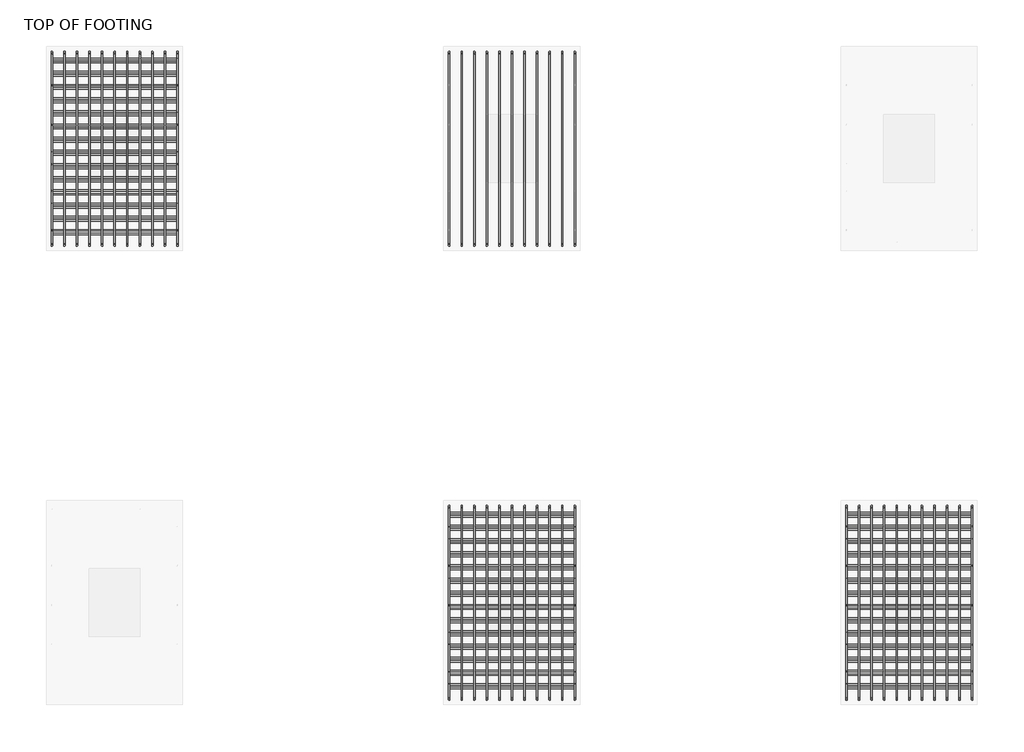
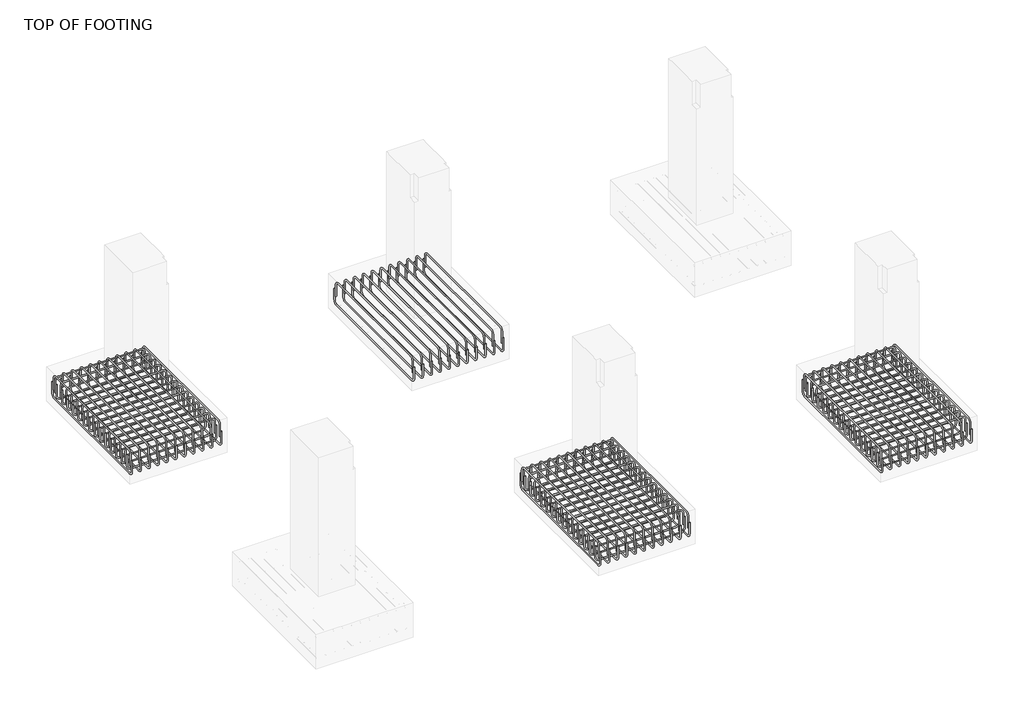
# One storey, part 5 of 11: 14 reinforcing bars.
"""IFC4 building model written with IfcOpenShell, lengths in millimetres."""

from ifc_helpers import new_model, si_unit, point, frame, origin, place, context, project, spatial, polyline, circle_curve, trimmed, segment, composite_curve, source, transform, mapped, element, save
from ifc_brep_helpers import swept_disk

model = new_model("IFC4")

# Units and contexts
model_context = context("Model", 3, world=origin())
ifc_project = project(units=[si_unit("LENGTHUNIT", "METRE", prefix="MILLI")], contexts=[model_context])

# Site, building, storey
site = spatial("IfcSite", under=ifc_project)
building = spatial("IfcBuilding", under=site)
storey = spatial("IfcBuildingStorey", under=building, Name="TOP OF FOOTING", Elevation=-1828.8)

# Reinforcing bars
placement = place(None, origin())
reinforcing_bar_shape = source(origin(), model_context, "Body", "SolidModel", [
    swept_disk(composite_curve([segment(polyline([(-8816.2384094, 14549.4712443, -2012.1658531), (-8816.2384094, 14549.4712443, -2159.4658531)]), True, "CONTINUOUS"), segment(trimmed(circle_curve(frame((-8816.2384094, 14595.8212443, -2159.4658531), z_axis=(1.0, 0.0, 0.0), x_axis=(0.0, -46.349999999998545, 0.0)), 46.35), [point((-8816.2384094, 14549.4712443, -2159.4658531))], [point((-8816.2384094, 14595.8212443, -2205.8158531))], True, "CARTESIAN"), True, "CONTINUOUS"), segment(polyline([(-8816.2384094, 14595.8212443, -2205.8158531), (-8816.2384094, 16210.4212443, -2205.8158531)]), True, "CONTINUOUS"), segment(trimmed(circle_curve(frame((-8816.2384094, 16210.4212443, -2159.4658531), z_axis=(1.0, 0.0, 0.0), x_axis=(0.0, 0.0, -46.34999999999991)), 46.35), [point((-8816.2384094, 16210.4212443, -2205.8158531))], [point((-8816.2384094, 16256.7712443, -2159.4658531))], True, "CARTESIAN"), True, "CONTINUOUS"), segment(polyline([(-8816.2384094, 16256.7712443, -2159.4658531), (-8816.2384094, 16256.7712443, -2012.1658531)]), True, "CONTINUOUS")], self_intersect=False), 6.35),
])
element("IfcReinforcingBar", 1, at=placement, inside=storey, context=model_context, shape_type="MappedRepresentation", body=[
    mapped(reinforcing_bar_shape, transform((0.0, 0.0, 0.0), x_axis=(1.0, 0.0, 0.0), y_axis=(0.0, 1.0, 0.0), z_axis=(0.0, 0.0, 1.0))),
    mapped(reinforcing_bar_shape, transform((-110.73, 0.0, 0.0), x_axis=(1.0, 0.0, 0.0), y_axis=(0.0, 1.0, 0.0), z_axis=(0.0, 0.0, 1.0))),
    mapped(reinforcing_bar_shape, transform((-221.46, 0.0, 0.0), x_axis=(1.0, 0.0, 0.0), y_axis=(0.0, 1.0, 0.0), z_axis=(0.0, 0.0, 1.0))),
    mapped(reinforcing_bar_shape, transform((-332.19, 0.0, 0.0), x_axis=(1.0, 0.0, 0.0), y_axis=(0.0, 1.0, 0.0), z_axis=(0.0, 0.0, 1.0))),
    mapped(reinforcing_bar_shape, transform((-442.92, 0.0, 0.0), x_axis=(1.0, 0.0, 0.0), y_axis=(0.0, 1.0, 0.0), z_axis=(0.0, 0.0, 1.0))),
    mapped(reinforcing_bar_shape, transform((-553.65, 0.0, 0.0), x_axis=(1.0, 0.0, 0.0), y_axis=(0.0, 1.0, 0.0), z_axis=(0.0, 0.0, 1.0))),
    mapped(reinforcing_bar_shape, transform((-664.38, 0.0, 0.0), x_axis=(1.0, 0.0, 0.0), y_axis=(0.0, 1.0, 0.0), z_axis=(0.0, 0.0, 1.0))),
    mapped(reinforcing_bar_shape, transform((-775.11, 0.0, 0.0), x_axis=(1.0, 0.0, 0.0), y_axis=(0.0, 1.0, 0.0), z_axis=(0.0, 0.0, 1.0))),
    mapped(reinforcing_bar_shape, transform((-885.84, 0.0, 0.0), x_axis=(1.0, 0.0, 0.0), y_axis=(0.0, 1.0, 0.0), z_axis=(0.0, 0.0, 1.0))),
    mapped(reinforcing_bar_shape, transform((-996.57, 0.0, 0.0), x_axis=(1.0, 0.0, 0.0), y_axis=(0.0, 1.0, 0.0), z_axis=(0.0, 0.0, 1.0))),
    mapped(reinforcing_bar_shape, transform((-1107.3, 0.0, 0.0), x_axis=(1.0, 0.0, 0.0), y_axis=(0.0, 1.0, 0.0), z_axis=(0.0, 0.0, 1.0))),
])
reinforcing_bar_2_shape = source(origin(), model_context, "Body", "SolidModel", [
    swept_disk(composite_curve([segment(polyline([(-9923.5384094, 14577.6603603, -2096.8914539), (-9923.5384094, 14577.6603603, -1949.5914539)]), True, "CONTINUOUS"), segment(trimmed(circle_curve(frame((-9923.5384094, 14624.0103603, -1949.5914539), z_axis=(-1.0, 0.0, 0.0), x_axis=(0.0, -46.350000000000364, 0.0)), 46.35), [point((-9923.5384094, 14577.6603603, -1949.5914539))], [point((-9923.5384094, 14624.0103603, -1903.2414539))], True, "CARTESIAN"), True, "CONTINUOUS"), segment(polyline([(-9923.5384094, 14624.0103603, -1903.2414539), (-9923.5384094, 16181.3238837, -1903.2414539)]), True, "CONTINUOUS"), segment(trimmed(circle_curve(frame((-9923.5384094, 16181.3238837, -1949.5914539), z_axis=(-1.0, 0.0, 0.0), x_axis=(0.0, 0.0, 46.350000000000136)), 46.35), [point((-9923.5384094, 16181.3238837, -1903.2414539))], [point((-9923.5384094, 16227.6738837, -1949.5914539))], True, "CARTESIAN"), True, "CONTINUOUS"), segment(polyline([(-9923.5384094, 16227.6738837, -1949.5914539), (-9923.5384094, 16227.6738837, -2096.8914539)]), True, "CONTINUOUS")], self_intersect=False), 6.35),
])
element("IfcReinforcingBar", 2, at=placement, inside=storey, context=model_context, shape_type="MappedRepresentation", body=[
    mapped(reinforcing_bar_2_shape, transform((0.0, 0.0, 0.0), x_axis=(1.0, 0.0, 0.0), y_axis=(0.0, 1.0, 0.0), z_axis=(0.0, 0.0, 1.0))),
    mapped(reinforcing_bar_2_shape, transform((110.73, 0.0, 0.0), x_axis=(1.0, 0.0, 0.0), y_axis=(0.0, 1.0, 0.0), z_axis=(0.0, 0.0, 1.0))),
    mapped(reinforcing_bar_2_shape, transform((221.46, 0.0, 0.0), x_axis=(1.0, 0.0, 0.0), y_axis=(0.0, 1.0, 0.0), z_axis=(0.0, 0.0, 1.0))),
    mapped(reinforcing_bar_2_shape, transform((332.19, 0.0, 0.0), x_axis=(1.0, 0.0, 0.0), y_axis=(0.0, 1.0, 0.0), z_axis=(0.0, 0.0, 1.0))),
    mapped(reinforcing_bar_2_shape, transform((442.92, 0.0, 0.0), x_axis=(1.0, 0.0, 0.0), y_axis=(0.0, 1.0, 0.0), z_axis=(0.0, 0.0, 1.0))),
    mapped(reinforcing_bar_2_shape, transform((553.65, 0.0, 0.0), x_axis=(1.0, 0.0, 0.0), y_axis=(0.0, 1.0, 0.0), z_axis=(0.0, 0.0, 1.0))),
    mapped(reinforcing_bar_2_shape, transform((664.38, 0.0, 0.0), x_axis=(1.0, 0.0, 0.0), y_axis=(0.0, 1.0, 0.0), z_axis=(0.0, 0.0, 1.0))),
    mapped(reinforcing_bar_2_shape, transform((775.11, 0.0, 0.0), x_axis=(1.0, 0.0, 0.0), y_axis=(0.0, 1.0, 0.0), z_axis=(0.0, 0.0, 1.0))),
    mapped(reinforcing_bar_2_shape, transform((885.84, 0.0, 0.0), x_axis=(1.0, 0.0, 0.0), y_axis=(0.0, 1.0, 0.0), z_axis=(0.0, 0.0, 1.0))),
    mapped(reinforcing_bar_2_shape, transform((996.57, 0.0, 0.0), x_axis=(1.0, 0.0, 0.0), y_axis=(0.0, 1.0, 0.0), z_axis=(0.0, 0.0, 1.0))),
    mapped(reinforcing_bar_2_shape, transform((1107.3, 0.0, 0.0), x_axis=(1.0, 0.0, 0.0), y_axis=(0.0, 1.0, 0.0), z_axis=(0.0, 0.0, 1.0))),
])
reinforcing_bar_3_shape = source(origin(), model_context, "Body", "SolidModel", [
    swept_disk(composite_curve([segment(polyline([(-9923.5384094, 14653.1930221, -1996.7664426), (-9923.5384094, 14653.1930221, -2144.0664426)]), True, "CONTINUOUS"), segment(trimmed(circle_curve(frame((-9877.1884094, 14653.1930221, -2144.0664426), z_axis=(0.0, -1.0, 0.0), x_axis=(-46.350000000000364, 0.0, 0.0)), 46.35), [point((-9923.5384094, 14653.1930221, -2144.0664426))], [point((-9877.1884094, 14653.1930221, -2190.4164426))], True, "CARTESIAN"), True, "CONTINUOUS"), segment(polyline([(-9877.1884094, 14653.1930221, -2190.4164426), (-8862.5884094, 14653.1930221, -2190.4164426)]), True, "CONTINUOUS"), segment(trimmed(circle_curve(frame((-8862.5884094, 14653.1930221, -2144.0664426), z_axis=(0.0, -1.0, 0.0), x_axis=(0.0, 0.0, -46.350000000000364)), 46.35), [point((-8862.5884094, 14653.1930221, -2190.4164426))], [point((-8816.2384094, 14653.1930221, -2144.0664426))], True, "CARTESIAN"), True, "CONTINUOUS"), segment(polyline([(-8816.2384094, 14653.1930221, -2144.0664426), (-8816.2384094, 14653.1930221, -1996.7664426)]), True, "CONTINUOUS")], self_intersect=False), 6.35),
])
element("IfcReinforcingBar", 3, at=placement, inside=storey, context=model_context, shape_type="MappedRepresentation", body=[
    mapped(reinforcing_bar_3_shape, transform((0.0, 0.0, 0.0), x_axis=(1.0, 0.0, 0.0), y_axis=(0.0, 1.0, 0.0), z_axis=(0.0, 0.0, 1.0))),
    mapped(reinforcing_bar_3_shape, transform((0.0, 116.2744005, 0.0), x_axis=(1.0, 0.0, 0.0), y_axis=(0.0, 1.0, 0.0), z_axis=(0.0, 0.0, 1.0))),
    mapped(reinforcing_bar_3_shape, transform((0.0, 232.5488009, 0.0), x_axis=(1.0, 0.0, 0.0), y_axis=(0.0, 1.0, 0.0), z_axis=(0.0, 0.0, 1.0))),
    mapped(reinforcing_bar_3_shape, transform((0.0, 348.8232014, 0.0), x_axis=(1.0, 0.0, 0.0), y_axis=(0.0, 1.0, 0.0), z_axis=(0.0, 0.0, 1.0))),
    mapped(reinforcing_bar_3_shape, transform((0.0, 465.0976018, 0.0), x_axis=(1.0, 0.0, 0.0), y_axis=(0.0, 1.0, 0.0), z_axis=(0.0, 0.0, 1.0))),
    mapped(reinforcing_bar_3_shape, transform((0.0, 581.3720023, 0.0), x_axis=(1.0, 0.0, 0.0), y_axis=(0.0, 1.0, 0.0), z_axis=(0.0, 0.0, 1.0))),
    mapped(reinforcing_bar_3_shape, transform((0.0, 697.6464027, 0.0), x_axis=(1.0, 0.0, 0.0), y_axis=(0.0, 1.0, 0.0), z_axis=(0.0, 0.0, 1.0))),
    mapped(reinforcing_bar_3_shape, transform((0.0, 813.9208032, 0.0), x_axis=(1.0, 0.0, 0.0), y_axis=(0.0, 1.0, 0.0), z_axis=(0.0, 0.0, 1.0))),
    mapped(reinforcing_bar_3_shape, transform((0.0, 930.1952036, 0.0), x_axis=(1.0, 0.0, 0.0), y_axis=(0.0, 1.0, 0.0), z_axis=(0.0, 0.0, 1.0))),
    mapped(reinforcing_bar_3_shape, transform((0.0, 1046.4696041, 0.0), x_axis=(1.0, 0.0, 0.0), y_axis=(0.0, 1.0, 0.0), z_axis=(0.0, 0.0, 1.0))),
    mapped(reinforcing_bar_3_shape, transform((0.0, 1162.7440045, 0.0), x_axis=(1.0, 0.0, 0.0), y_axis=(0.0, 1.0, 0.0), z_axis=(0.0, 0.0, 1.0))),
    mapped(reinforcing_bar_3_shape, transform((0.0, 1279.018405, 0.0), x_axis=(1.0, 0.0, 0.0), y_axis=(0.0, 1.0, 0.0), z_axis=(0.0, 0.0, 1.0))),
    mapped(reinforcing_bar_3_shape, transform((0.0, 1395.2928054, 0.0), x_axis=(1.0, 0.0, 0.0), y_axis=(0.0, 1.0, 0.0), z_axis=(0.0, 0.0, 1.0))),
    mapped(reinforcing_bar_3_shape, transform((0.0, 1511.5672059, 0.0), x_axis=(1.0, 0.0, 0.0), y_axis=(0.0, 1.0, 0.0), z_axis=(0.0, 0.0, 1.0))),
])
reinforcing_bar_4_shape = source(origin(), model_context, "Body", "SolidModel", [
    swept_disk(composite_curve([segment(polyline([(-9923.5384094, 16194.4257435, -2114.1958609), (-9923.5384094, 16194.4257435, -1966.8958609)]), True, "CONTINUOUS"), segment(trimmed(circle_curve(frame((-9877.1884094, 16194.4257435, -1966.8958609), z_axis=(0.0, 1.0, 0.0), x_axis=(-46.350000000000364, 0.0, 0.0)), 46.35), [point((-9923.5384094, 16194.4257435, -1966.8958609))], [point((-9877.1884094, 16194.4257435, -1920.5458609))], True, "CARTESIAN"), True, "CONTINUOUS"), segment(polyline([(-9877.1884094, 16194.4257435, -1920.5458609), (-8862.5884094, 16194.4257435, -1920.5458609)]), True, "CONTINUOUS"), segment(trimmed(circle_curve(frame((-8862.5884094, 16194.4257435, -1966.8958609), z_axis=(0.0, 1.0, 0.0), x_axis=(0.0, 0.0, 46.34999999999991)), 46.35), [point((-8862.5884094, 16194.4257435, -1920.5458609))], [point((-8816.2384094, 16194.4257435, -1966.8958609))], True, "CARTESIAN"), True, "CONTINUOUS"), segment(polyline([(-8816.2384094, 16194.4257435, -1966.8958609), (-8816.2384094, 16194.4257435, -2114.1958609)]), True, "CONTINUOUS")], self_intersect=False), 6.35),
])
element("IfcReinforcingBar", 4, at=placement, inside=storey, context=model_context, shape_type="MappedRepresentation", body=[
    mapped(reinforcing_bar_4_shape, transform((0.0, 0.0, 0.0), x_axis=(1.0, 0.0, 0.0), y_axis=(0.0, 1.0, 0.0), z_axis=(0.0, 0.0, 1.0))),
    mapped(reinforcing_bar_4_shape, transform((0.0, -116.1057918, 0.0), x_axis=(1.0, 0.0, 0.0), y_axis=(0.0, 1.0, 0.0), z_axis=(0.0, 0.0, 1.0))),
    mapped(reinforcing_bar_4_shape, transform((0.0, -232.2115836, 0.0), x_axis=(1.0, 0.0, 0.0), y_axis=(0.0, 1.0, 0.0), z_axis=(0.0, 0.0, 1.0))),
    mapped(reinforcing_bar_4_shape, transform((0.0, -348.3173754, 0.0), x_axis=(1.0, 0.0, 0.0), y_axis=(0.0, 1.0, 0.0), z_axis=(0.0, 0.0, 1.0))),
    mapped(reinforcing_bar_4_shape, transform((0.0, -464.4231672, 0.0), x_axis=(1.0, 0.0, 0.0), y_axis=(0.0, 1.0, 0.0), z_axis=(0.0, 0.0, 1.0))),
    mapped(reinforcing_bar_4_shape, transform((0.0, -580.528959, 0.0), x_axis=(1.0, 0.0, 0.0), y_axis=(0.0, 1.0, 0.0), z_axis=(0.0, 0.0, 1.0))),
    mapped(reinforcing_bar_4_shape, transform((0.0, -696.6347508, 0.0), x_axis=(1.0, 0.0, 0.0), y_axis=(0.0, 1.0, 0.0), z_axis=(0.0, 0.0, 1.0))),
    mapped(reinforcing_bar_4_shape, transform((0.0, -812.7405426, 0.0), x_axis=(1.0, 0.0, 0.0), y_axis=(0.0, 1.0, 0.0), z_axis=(0.0, 0.0, 1.0))),
    mapped(reinforcing_bar_4_shape, transform((0.0, -928.8463344, 0.0), x_axis=(1.0, 0.0, 0.0), y_axis=(0.0, 1.0, 0.0), z_axis=(0.0, 0.0, 1.0))),
    mapped(reinforcing_bar_4_shape, transform((0.0, -1044.9521262, 0.0), x_axis=(1.0, 0.0, 0.0), y_axis=(0.0, 1.0, 0.0), z_axis=(0.0, 0.0, 1.0))),
    mapped(reinforcing_bar_4_shape, transform((0.0, -1161.057918, 0.0), x_axis=(1.0, 0.0, 0.0), y_axis=(0.0, 1.0, 0.0), z_axis=(0.0, 0.0, 1.0))),
    mapped(reinforcing_bar_4_shape, transform((0.0, -1277.1637098, 0.0), x_axis=(1.0, 0.0, 0.0), y_axis=(0.0, 1.0, 0.0), z_axis=(0.0, 0.0, 1.0))),
    mapped(reinforcing_bar_4_shape, transform((0.0, -1393.2695016, 0.0), x_axis=(1.0, 0.0, 0.0), y_axis=(0.0, 1.0, 0.0), z_axis=(0.0, 0.0, 1.0))),
    mapped(reinforcing_bar_4_shape, transform((0.0, -1509.3752934, 0.0), x_axis=(1.0, 0.0, 0.0), y_axis=(0.0, 1.0, 0.0), z_axis=(0.0, 0.0, 1.0))),
])
reinforcing_bar_5_shape = source(origin(), model_context, "Body", "SolidModel", [
    swept_disk(composite_curve([segment(polyline([(-5316.2384094, 14549.4712443, -2012.1658531), (-5316.2384094, 14549.4712443, -2159.4658531)]), True, "CONTINUOUS"), segment(trimmed(circle_curve(frame((-5316.2384094, 14595.8212443, -2159.4658531), z_axis=(1.0, 0.0, 0.0), x_axis=(0.0, -46.349999999998545, 0.0)), 46.35), [point((-5316.2384094, 14549.4712443, -2159.4658531))], [point((-5316.2384094, 14595.8212443, -2205.8158531))], True, "CARTESIAN"), True, "CONTINUOUS"), segment(polyline([(-5316.2384094, 14595.8212443, -2205.8158531), (-5316.2384094, 16210.4212443, -2205.8158531)]), True, "CONTINUOUS"), segment(trimmed(circle_curve(frame((-5316.2384094, 16210.4212443, -2159.4658531), z_axis=(1.0, 0.0, 0.0), x_axis=(0.0, 0.0, -46.34999999999991)), 46.35), [point((-5316.2384094, 16210.4212443, -2205.8158531))], [point((-5316.2384094, 16256.7712443, -2159.4658531))], True, "CARTESIAN"), True, "CONTINUOUS"), segment(polyline([(-5316.2384094, 16256.7712443, -2159.4658531), (-5316.2384094, 16256.7712443, -2012.1658531)]), True, "CONTINUOUS")], self_intersect=False), 6.35),
])
element("IfcReinforcingBar", 5, at=placement, inside=storey, context=model_context, shape_type="MappedRepresentation", body=[
    mapped(reinforcing_bar_5_shape, transform((0.0, 0.0, 0.0), x_axis=(1.0, 0.0, 0.0), y_axis=(0.0, 1.0, 0.0), z_axis=(0.0, 0.0, 1.0))),
    mapped(reinforcing_bar_5_shape, transform((-110.73, 0.0, 0.0), x_axis=(1.0, 0.0, 0.0), y_axis=(0.0, 1.0, 0.0), z_axis=(0.0, 0.0, 1.0))),
    mapped(reinforcing_bar_5_shape, transform((-221.46, 0.0, 0.0), x_axis=(1.0, 0.0, 0.0), y_axis=(0.0, 1.0, 0.0), z_axis=(0.0, 0.0, 1.0))),
    mapped(reinforcing_bar_5_shape, transform((-332.19, 0.0, 0.0), x_axis=(1.0, 0.0, 0.0), y_axis=(0.0, 1.0, 0.0), z_axis=(0.0, 0.0, 1.0))),
    mapped(reinforcing_bar_5_shape, transform((-442.92, 0.0, 0.0), x_axis=(1.0, 0.0, 0.0), y_axis=(0.0, 1.0, 0.0), z_axis=(0.0, 0.0, 1.0))),
    mapped(reinforcing_bar_5_shape, transform((-553.65, 0.0, 0.0), x_axis=(1.0, 0.0, 0.0), y_axis=(0.0, 1.0, 0.0), z_axis=(0.0, 0.0, 1.0))),
    mapped(reinforcing_bar_5_shape, transform((-664.38, 0.0, 0.0), x_axis=(1.0, 0.0, 0.0), y_axis=(0.0, 1.0, 0.0), z_axis=(0.0, 0.0, 1.0))),
    mapped(reinforcing_bar_5_shape, transform((-775.11, 0.0, 0.0), x_axis=(1.0, 0.0, 0.0), y_axis=(0.0, 1.0, 0.0), z_axis=(0.0, 0.0, 1.0))),
    mapped(reinforcing_bar_5_shape, transform((-885.84, 0.0, 0.0), x_axis=(1.0, 0.0, 0.0), y_axis=(0.0, 1.0, 0.0), z_axis=(0.0, 0.0, 1.0))),
    mapped(reinforcing_bar_5_shape, transform((-996.57, 0.0, 0.0), x_axis=(1.0, 0.0, 0.0), y_axis=(0.0, 1.0, 0.0), z_axis=(0.0, 0.0, 1.0))),
    mapped(reinforcing_bar_5_shape, transform((-1107.3, 0.0, 0.0), x_axis=(1.0, 0.0, 0.0), y_axis=(0.0, 1.0, 0.0), z_axis=(0.0, 0.0, 1.0))),
])
reinforcing_bar_6_shape = source(origin(), model_context, "Body", "SolidModel", [
    swept_disk(composite_curve([segment(polyline([(-6423.5384094, 14577.6603603, -2096.8914539), (-6423.5384094, 14577.6603603, -1949.5914539)]), True, "CONTINUOUS"), segment(trimmed(circle_curve(frame((-6423.5384094, 14624.0103603, -1949.5914539), z_axis=(-1.0, 0.0, 0.0), x_axis=(0.0, -46.350000000000364, 0.0)), 46.35), [point((-6423.5384094, 14577.6603603, -1949.5914539))], [point((-6423.5384094, 14624.0103603, -1903.2414539))], True, "CARTESIAN"), True, "CONTINUOUS"), segment(polyline([(-6423.5384094, 14624.0103603, -1903.2414539), (-6423.5384094, 16181.3238837, -1903.2414539)]), True, "CONTINUOUS"), segment(trimmed(circle_curve(frame((-6423.5384094, 16181.3238837, -1949.5914539), z_axis=(-1.0, 0.0, 0.0), x_axis=(0.0, 0.0, 46.350000000000136)), 46.35), [point((-6423.5384094, 16181.3238837, -1903.2414539))], [point((-6423.5384094, 16227.6738837, -1949.5914539))], True, "CARTESIAN"), True, "CONTINUOUS"), segment(polyline([(-6423.5384094, 16227.6738837, -1949.5914539), (-6423.5384094, 16227.6738837, -2096.8914539)]), True, "CONTINUOUS")], self_intersect=False), 6.35),
])
element("IfcReinforcingBar", 6, at=placement, inside=storey, context=model_context, shape_type="MappedRepresentation", body=[
    mapped(reinforcing_bar_6_shape, transform((0.0, 0.0, 0.0), x_axis=(1.0, 0.0, 0.0), y_axis=(0.0, 1.0, 0.0), z_axis=(0.0, 0.0, 1.0))),
    mapped(reinforcing_bar_6_shape, transform((110.73, 0.0, 0.0), x_axis=(1.0, 0.0, 0.0), y_axis=(0.0, 1.0, 0.0), z_axis=(0.0, 0.0, 1.0))),
    mapped(reinforcing_bar_6_shape, transform((221.46, 0.0, 0.0), x_axis=(1.0, 0.0, 0.0), y_axis=(0.0, 1.0, 0.0), z_axis=(0.0, 0.0, 1.0))),
    mapped(reinforcing_bar_6_shape, transform((332.19, 0.0, 0.0), x_axis=(1.0, 0.0, 0.0), y_axis=(0.0, 1.0, 0.0), z_axis=(0.0, 0.0, 1.0))),
    mapped(reinforcing_bar_6_shape, transform((442.92, 0.0, 0.0), x_axis=(1.0, 0.0, 0.0), y_axis=(0.0, 1.0, 0.0), z_axis=(0.0, 0.0, 1.0))),
    mapped(reinforcing_bar_6_shape, transform((553.65, 0.0, 0.0), x_axis=(1.0, 0.0, 0.0), y_axis=(0.0, 1.0, 0.0), z_axis=(0.0, 0.0, 1.0))),
    mapped(reinforcing_bar_6_shape, transform((664.38, 0.0, 0.0), x_axis=(1.0, 0.0, 0.0), y_axis=(0.0, 1.0, 0.0), z_axis=(0.0, 0.0, 1.0))),
    mapped(reinforcing_bar_6_shape, transform((775.11, 0.0, 0.0), x_axis=(1.0, 0.0, 0.0), y_axis=(0.0, 1.0, 0.0), z_axis=(0.0, 0.0, 1.0))),
    mapped(reinforcing_bar_6_shape, transform((885.84, 0.0, 0.0), x_axis=(1.0, 0.0, 0.0), y_axis=(0.0, 1.0, 0.0), z_axis=(0.0, 0.0, 1.0))),
    mapped(reinforcing_bar_6_shape, transform((996.57, 0.0, 0.0), x_axis=(1.0, 0.0, 0.0), y_axis=(0.0, 1.0, 0.0), z_axis=(0.0, 0.0, 1.0))),
    mapped(reinforcing_bar_6_shape, transform((1107.3, 0.0, 0.0), x_axis=(1.0, 0.0, 0.0), y_axis=(0.0, 1.0, 0.0), z_axis=(0.0, 0.0, 1.0))),
])
reinforcing_bar_7_shape = source(origin(), model_context, "Body", "SolidModel", [
    swept_disk(composite_curve([segment(polyline([(-1816.2384094, 10549.4712443, -2012.1658531), (-1816.2384094, 10549.4712443, -2159.4658531)]), True, "CONTINUOUS"), segment(trimmed(circle_curve(frame((-1816.2384094, 10595.8212443, -2159.4658531), z_axis=(1.0, 0.0, 0.0), x_axis=(0.0, -46.349999999998545, 0.0)), 46.35), [point((-1816.2384094, 10549.4712443, -2159.4658531))], [point((-1816.2384094, 10595.8212443, -2205.8158531))], True, "CARTESIAN"), True, "CONTINUOUS"), segment(polyline([(-1816.2384094, 10595.8212443, -2205.8158531), (-1816.2384094, 12210.4212443, -2205.8158531)]), True, "CONTINUOUS"), segment(trimmed(circle_curve(frame((-1816.2384094, 12210.4212443, -2159.4658531), z_axis=(1.0, 0.0, 0.0), x_axis=(0.0, 0.0, -46.34999999999991)), 46.35), [point((-1816.2384094, 12210.4212443, -2205.8158531))], [point((-1816.2384094, 12256.7712443, -2159.4658531))], True, "CARTESIAN"), True, "CONTINUOUS"), segment(polyline([(-1816.2384094, 12256.7712443, -2159.4658531), (-1816.2384094, 12256.7712443, -2012.1658531)]), True, "CONTINUOUS")], self_intersect=False), 6.35),
])
element("IfcReinforcingBar", 7, at=placement, inside=storey, context=model_context, shape_type="MappedRepresentation", body=[
    mapped(reinforcing_bar_7_shape, transform((0.0, 0.0, 0.0), x_axis=(1.0, 0.0, 0.0), y_axis=(0.0, 1.0, 0.0), z_axis=(0.0, 0.0, 1.0))),
    mapped(reinforcing_bar_7_shape, transform((-110.73, 0.0, 0.0), x_axis=(1.0, 0.0, 0.0), y_axis=(0.0, 1.0, 0.0), z_axis=(0.0, 0.0, 1.0))),
    mapped(reinforcing_bar_7_shape, transform((-221.46, 0.0, 0.0), x_axis=(1.0, 0.0, 0.0), y_axis=(0.0, 1.0, 0.0), z_axis=(0.0, 0.0, 1.0))),
    mapped(reinforcing_bar_7_shape, transform((-332.19, 0.0, 0.0), x_axis=(1.0, 0.0, 0.0), y_axis=(0.0, 1.0, 0.0), z_axis=(0.0, 0.0, 1.0))),
    mapped(reinforcing_bar_7_shape, transform((-442.92, 0.0, 0.0), x_axis=(1.0, 0.0, 0.0), y_axis=(0.0, 1.0, 0.0), z_axis=(0.0, 0.0, 1.0))),
    mapped(reinforcing_bar_7_shape, transform((-553.65, 0.0, 0.0), x_axis=(1.0, 0.0, 0.0), y_axis=(0.0, 1.0, 0.0), z_axis=(0.0, 0.0, 1.0))),
    mapped(reinforcing_bar_7_shape, transform((-664.38, 0.0, 0.0), x_axis=(1.0, 0.0, 0.0), y_axis=(0.0, 1.0, 0.0), z_axis=(0.0, 0.0, 1.0))),
    mapped(reinforcing_bar_7_shape, transform((-775.11, 0.0, 0.0), x_axis=(1.0, 0.0, 0.0), y_axis=(0.0, 1.0, 0.0), z_axis=(0.0, 0.0, 1.0))),
    mapped(reinforcing_bar_7_shape, transform((-885.84, 0.0, 0.0), x_axis=(1.0, 0.0, 0.0), y_axis=(0.0, 1.0, 0.0), z_axis=(0.0, 0.0, 1.0))),
    mapped(reinforcing_bar_7_shape, transform((-996.57, 0.0, 0.0), x_axis=(1.0, 0.0, 0.0), y_axis=(0.0, 1.0, 0.0), z_axis=(0.0, 0.0, 1.0))),
    mapped(reinforcing_bar_7_shape, transform((-1107.3, 0.0, 0.0), x_axis=(1.0, 0.0, 0.0), y_axis=(0.0, 1.0, 0.0), z_axis=(0.0, 0.0, 1.0))),
])
reinforcing_bar_8_shape = source(origin(), model_context, "Body", "SolidModel", [
    swept_disk(composite_curve([segment(polyline([(-2923.5384094, 10577.6603603, -2096.8914539), (-2923.5384094, 10577.6603603, -1949.5914539)]), True, "CONTINUOUS"), segment(trimmed(circle_curve(frame((-2923.5384094, 10624.0103603, -1949.5914539), z_axis=(-1.0, 0.0, 0.0), x_axis=(0.0, -46.350000000000364, 0.0)), 46.35), [point((-2923.5384094, 10577.6603603, -1949.5914539))], [point((-2923.5384094, 10624.0103603, -1903.2414539))], True, "CARTESIAN"), True, "CONTINUOUS"), segment(polyline([(-2923.5384094, 10624.0103603, -1903.2414539), (-2923.5384094, 12181.3238837, -1903.2414539)]), True, "CONTINUOUS"), segment(trimmed(circle_curve(frame((-2923.5384094, 12181.3238837, -1949.5914539), z_axis=(-1.0, 0.0, 0.0), x_axis=(0.0, 0.0, 46.350000000000136)), 46.35), [point((-2923.5384094, 12181.3238837, -1903.2414539))], [point((-2923.5384094, 12227.6738837, -1949.5914539))], True, "CARTESIAN"), True, "CONTINUOUS"), segment(polyline([(-2923.5384094, 12227.6738837, -1949.5914539), (-2923.5384094, 12227.6738837, -2096.8914539)]), True, "CONTINUOUS")], self_intersect=False), 6.35),
])
element("IfcReinforcingBar", 8, at=placement, inside=storey, context=model_context, shape_type="MappedRepresentation", body=[
    mapped(reinforcing_bar_8_shape, transform((0.0, 0.0, 0.0), x_axis=(1.0, 0.0, 0.0), y_axis=(0.0, 1.0, 0.0), z_axis=(0.0, 0.0, 1.0))),
    mapped(reinforcing_bar_8_shape, transform((110.73, 0.0, 0.0), x_axis=(1.0, 0.0, 0.0), y_axis=(0.0, 1.0, 0.0), z_axis=(0.0, 0.0, 1.0))),
    mapped(reinforcing_bar_8_shape, transform((221.46, 0.0, 0.0), x_axis=(1.0, 0.0, 0.0), y_axis=(0.0, 1.0, 0.0), z_axis=(0.0, 0.0, 1.0))),
    mapped(reinforcing_bar_8_shape, transform((332.19, 0.0, 0.0), x_axis=(1.0, 0.0, 0.0), y_axis=(0.0, 1.0, 0.0), z_axis=(0.0, 0.0, 1.0))),
    mapped(reinforcing_bar_8_shape, transform((442.92, 0.0, 0.0), x_axis=(1.0, 0.0, 0.0), y_axis=(0.0, 1.0, 0.0), z_axis=(0.0, 0.0, 1.0))),
    mapped(reinforcing_bar_8_shape, transform((553.65, 0.0, 0.0), x_axis=(1.0, 0.0, 0.0), y_axis=(0.0, 1.0, 0.0), z_axis=(0.0, 0.0, 1.0))),
    mapped(reinforcing_bar_8_shape, transform((664.38, 0.0, 0.0), x_axis=(1.0, 0.0, 0.0), y_axis=(0.0, 1.0, 0.0), z_axis=(0.0, 0.0, 1.0))),
    mapped(reinforcing_bar_8_shape, transform((775.11, 0.0, 0.0), x_axis=(1.0, 0.0, 0.0), y_axis=(0.0, 1.0, 0.0), z_axis=(0.0, 0.0, 1.0))),
    mapped(reinforcing_bar_8_shape, transform((885.84, 0.0, 0.0), x_axis=(1.0, 0.0, 0.0), y_axis=(0.0, 1.0, 0.0), z_axis=(0.0, 0.0, 1.0))),
    mapped(reinforcing_bar_8_shape, transform((996.57, 0.0, 0.0), x_axis=(1.0, 0.0, 0.0), y_axis=(0.0, 1.0, 0.0), z_axis=(0.0, 0.0, 1.0))),
    mapped(reinforcing_bar_8_shape, transform((1107.3, 0.0, 0.0), x_axis=(1.0, 0.0, 0.0), y_axis=(0.0, 1.0, 0.0), z_axis=(0.0, 0.0, 1.0))),
])
reinforcing_bar_9_shape = source(origin(), model_context, "Body", "SolidModel", [
    swept_disk(composite_curve([segment(polyline([(-2923.5384094, 10653.1930221, -1996.7664426), (-2923.5384094, 10653.1930221, -2144.0664426)]), True, "CONTINUOUS"), segment(trimmed(circle_curve(frame((-2877.1884094, 10653.1930221, -2144.0664426), z_axis=(0.0, -1.0, 0.0), x_axis=(-46.34999999999991, 0.0, 0.0)), 46.35), [point((-2923.5384094, 10653.1930221, -2144.0664426))], [point((-2877.1884094, 10653.1930221, -2190.4164426))], True, "CARTESIAN"), True, "CONTINUOUS"), segment(polyline([(-2877.1884094, 10653.1930221, -2190.4164426), (-1862.5884094, 10653.1930221, -2190.4164426)]), True, "CONTINUOUS"), segment(trimmed(circle_curve(frame((-1862.5884094, 10653.1930221, -2144.0664426), z_axis=(0.0, -1.0, 0.0), x_axis=(0.0, 0.0, -46.350000000000364)), 46.35), [point((-1862.5884094, 10653.1930221, -2190.4164426))], [point((-1816.2384094, 10653.1930221, -2144.0664426))], True, "CARTESIAN"), True, "CONTINUOUS"), segment(polyline([(-1816.2384094, 10653.1930221, -2144.0664426), (-1816.2384094, 10653.1930221, -1996.7664426)]), True, "CONTINUOUS")], self_intersect=False), 6.35),
])
element("IfcReinforcingBar", 9, at=placement, inside=storey, context=model_context, shape_type="MappedRepresentation", body=[
    mapped(reinforcing_bar_9_shape, transform((0.0, 0.0, 0.0), x_axis=(1.0, 0.0, 0.0), y_axis=(0.0, 1.0, 0.0), z_axis=(0.0, 0.0, 1.0))),
    mapped(reinforcing_bar_9_shape, transform((0.0, 116.2744005, 0.0), x_axis=(1.0, 0.0, 0.0), y_axis=(0.0, 1.0, 0.0), z_axis=(0.0, 0.0, 1.0))),
    mapped(reinforcing_bar_9_shape, transform((0.0, 232.5488009, 0.0), x_axis=(1.0, 0.0, 0.0), y_axis=(0.0, 1.0, 0.0), z_axis=(0.0, 0.0, 1.0))),
    mapped(reinforcing_bar_9_shape, transform((0.0, 348.8232014, 0.0), x_axis=(1.0, 0.0, 0.0), y_axis=(0.0, 1.0, 0.0), z_axis=(0.0, 0.0, 1.0))),
    mapped(reinforcing_bar_9_shape, transform((0.0, 465.0976018, 0.0), x_axis=(1.0, 0.0, 0.0), y_axis=(0.0, 1.0, 0.0), z_axis=(0.0, 0.0, 1.0))),
    mapped(reinforcing_bar_9_shape, transform((0.0, 581.3720023, 0.0), x_axis=(1.0, 0.0, 0.0), y_axis=(0.0, 1.0, 0.0), z_axis=(0.0, 0.0, 1.0))),
    mapped(reinforcing_bar_9_shape, transform((0.0, 697.6464027, 0.0), x_axis=(1.0, 0.0, 0.0), y_axis=(0.0, 1.0, 0.0), z_axis=(0.0, 0.0, 1.0))),
    mapped(reinforcing_bar_9_shape, transform((0.0, 813.9208032, 0.0), x_axis=(1.0, 0.0, 0.0), y_axis=(0.0, 1.0, 0.0), z_axis=(0.0, 0.0, 1.0))),
    mapped(reinforcing_bar_9_shape, transform((0.0, 930.1952036, 0.0), x_axis=(1.0, 0.0, 0.0), y_axis=(0.0, 1.0, 0.0), z_axis=(0.0, 0.0, 1.0))),
    mapped(reinforcing_bar_9_shape, transform((0.0, 1046.4696041, 0.0), x_axis=(1.0, 0.0, 0.0), y_axis=(0.0, 1.0, 0.0), z_axis=(0.0, 0.0, 1.0))),
    mapped(reinforcing_bar_9_shape, transform((0.0, 1162.7440045, 0.0), x_axis=(1.0, 0.0, 0.0), y_axis=(0.0, 1.0, 0.0), z_axis=(0.0, 0.0, 1.0))),
    mapped(reinforcing_bar_9_shape, transform((0.0, 1279.018405, 0.0), x_axis=(1.0, 0.0, 0.0), y_axis=(0.0, 1.0, 0.0), z_axis=(0.0, 0.0, 1.0))),
    mapped(reinforcing_bar_9_shape, transform((0.0, 1395.2928054, 0.0), x_axis=(1.0, 0.0, 0.0), y_axis=(0.0, 1.0, 0.0), z_axis=(0.0, 0.0, 1.0))),
    mapped(reinforcing_bar_9_shape, transform((0.0, 1511.5672059, 0.0), x_axis=(1.0, 0.0, 0.0), y_axis=(0.0, 1.0, 0.0), z_axis=(0.0, 0.0, 1.0))),
])
reinforcing_bar_10_shape = source(origin(), model_context, "Body", "SolidModel", [
    swept_disk(composite_curve([segment(polyline([(-2923.5384094, 12194.4257435, -2114.1958609), (-2923.5384094, 12194.4257435, -1966.8958609)]), True, "CONTINUOUS"), segment(trimmed(circle_curve(frame((-2877.1884094, 12194.4257435, -1966.8958609), z_axis=(0.0, 1.0, 0.0), x_axis=(-46.34999999999991, 0.0, 0.0)), 46.35), [point((-2923.5384094, 12194.4257435, -1966.8958609))], [point((-2877.1884094, 12194.4257435, -1920.5458609))], True, "CARTESIAN"), True, "CONTINUOUS"), segment(polyline([(-2877.1884094, 12194.4257435, -1920.5458609), (-1862.5884094, 12194.4257435, -1920.5458609)]), True, "CONTINUOUS"), segment(trimmed(circle_curve(frame((-1862.5884094, 12194.4257435, -1966.8958609), z_axis=(0.0, 1.0, 0.0), x_axis=(0.0, 0.0, 46.34999999999991)), 46.35), [point((-1862.5884094, 12194.4257435, -1920.5458609))], [point((-1816.2384094, 12194.4257435, -1966.8958609))], True, "CARTESIAN"), True, "CONTINUOUS"), segment(polyline([(-1816.2384094, 12194.4257435, -1966.8958609), (-1816.2384094, 12194.4257435, -2114.1958609)]), True, "CONTINUOUS")], self_intersect=False), 6.35),
])
element("IfcReinforcingBar", 10, at=placement, inside=storey, context=model_context, shape_type="MappedRepresentation", body=[
    mapped(reinforcing_bar_10_shape, transform((0.0, 0.0, 0.0), x_axis=(1.0, 0.0, 0.0), y_axis=(0.0, 1.0, 0.0), z_axis=(0.0, 0.0, 1.0))),
    mapped(reinforcing_bar_10_shape, transform((0.0, -116.1057918, 0.0), x_axis=(1.0, 0.0, 0.0), y_axis=(0.0, 1.0, 0.0), z_axis=(0.0, 0.0, 1.0))),
    mapped(reinforcing_bar_10_shape, transform((0.0, -232.2115836, 0.0), x_axis=(1.0, 0.0, 0.0), y_axis=(0.0, 1.0, 0.0), z_axis=(0.0, 0.0, 1.0))),
    mapped(reinforcing_bar_10_shape, transform((0.0, -348.3173754, 0.0), x_axis=(1.0, 0.0, 0.0), y_axis=(0.0, 1.0, 0.0), z_axis=(0.0, 0.0, 1.0))),
    mapped(reinforcing_bar_10_shape, transform((0.0, -464.4231672, 0.0), x_axis=(1.0, 0.0, 0.0), y_axis=(0.0, 1.0, 0.0), z_axis=(0.0, 0.0, 1.0))),
    mapped(reinforcing_bar_10_shape, transform((0.0, -580.528959, 0.0), x_axis=(1.0, 0.0, 0.0), y_axis=(0.0, 1.0, 0.0), z_axis=(0.0, 0.0, 1.0))),
    mapped(reinforcing_bar_10_shape, transform((0.0, -696.6347508, 0.0), x_axis=(1.0, 0.0, 0.0), y_axis=(0.0, 1.0, 0.0), z_axis=(0.0, 0.0, 1.0))),
    mapped(reinforcing_bar_10_shape, transform((0.0, -812.7405426, 0.0), x_axis=(1.0, 0.0, 0.0), y_axis=(0.0, 1.0, 0.0), z_axis=(0.0, 0.0, 1.0))),
    mapped(reinforcing_bar_10_shape, transform((0.0, -928.8463344, 0.0), x_axis=(1.0, 0.0, 0.0), y_axis=(0.0, 1.0, 0.0), z_axis=(0.0, 0.0, 1.0))),
    mapped(reinforcing_bar_10_shape, transform((0.0, -1044.9521262, 0.0), x_axis=(1.0, 0.0, 0.0), y_axis=(0.0, 1.0, 0.0), z_axis=(0.0, 0.0, 1.0))),
    mapped(reinforcing_bar_10_shape, transform((0.0, -1161.057918, 0.0), x_axis=(1.0, 0.0, 0.0), y_axis=(0.0, 1.0, 0.0), z_axis=(0.0, 0.0, 1.0))),
    mapped(reinforcing_bar_10_shape, transform((0.0, -1277.1637098, 0.0), x_axis=(1.0, 0.0, 0.0), y_axis=(0.0, 1.0, 0.0), z_axis=(0.0, 0.0, 1.0))),
    mapped(reinforcing_bar_10_shape, transform((0.0, -1393.2695016, 0.0), x_axis=(1.0, 0.0, 0.0), y_axis=(0.0, 1.0, 0.0), z_axis=(0.0, 0.0, 1.0))),
    mapped(reinforcing_bar_10_shape, transform((0.0, -1509.3752934, 0.0), x_axis=(1.0, 0.0, 0.0), y_axis=(0.0, 1.0, 0.0), z_axis=(0.0, 0.0, 1.0))),
])
reinforcing_bar_11_shape = source(origin(), model_context, "Body", "SolidModel", [
    swept_disk(composite_curve([segment(polyline([(-5316.2384094, 10549.4712443, -2012.1658531), (-5316.2384094, 10549.4712443, -2159.4658531)]), True, "CONTINUOUS"), segment(trimmed(circle_curve(frame((-5316.2384094, 10595.8212443, -2159.4658531), z_axis=(1.0, 0.0, 0.0), x_axis=(0.0, -46.349999999998545, 0.0)), 46.35), [point((-5316.2384094, 10549.4712443, -2159.4658531))], [point((-5316.2384094, 10595.8212443, -2205.8158531))], True, "CARTESIAN"), True, "CONTINUOUS"), segment(polyline([(-5316.2384094, 10595.8212443, -2205.8158531), (-5316.2384094, 12210.4212443, -2205.8158531)]), True, "CONTINUOUS"), segment(trimmed(circle_curve(frame((-5316.2384094, 12210.4212443, -2159.4658531), z_axis=(1.0, 0.0, 0.0), x_axis=(0.0, 0.0, -46.34999999999991)), 46.35), [point((-5316.2384094, 12210.4212443, -2205.8158531))], [point((-5316.2384094, 12256.7712443, -2159.4658531))], True, "CARTESIAN"), True, "CONTINUOUS"), segment(polyline([(-5316.2384094, 12256.7712443, -2159.4658531), (-5316.2384094, 12256.7712443, -2012.1658531)]), True, "CONTINUOUS")], self_intersect=False), 6.35),
])
element("IfcReinforcingBar", 11, at=placement, inside=storey, context=model_context, shape_type="MappedRepresentation", body=[
    mapped(reinforcing_bar_11_shape, transform((0.0, 0.0, 0.0), x_axis=(1.0, 0.0, 0.0), y_axis=(0.0, 1.0, 0.0), z_axis=(0.0, 0.0, 1.0))),
    mapped(reinforcing_bar_11_shape, transform((-110.73, 0.0, 0.0), x_axis=(1.0, 0.0, 0.0), y_axis=(0.0, 1.0, 0.0), z_axis=(0.0, 0.0, 1.0))),
    mapped(reinforcing_bar_11_shape, transform((-221.46, 0.0, 0.0), x_axis=(1.0, 0.0, 0.0), y_axis=(0.0, 1.0, 0.0), z_axis=(0.0, 0.0, 1.0))),
    mapped(reinforcing_bar_11_shape, transform((-332.19, 0.0, 0.0), x_axis=(1.0, 0.0, 0.0), y_axis=(0.0, 1.0, 0.0), z_axis=(0.0, 0.0, 1.0))),
    mapped(reinforcing_bar_11_shape, transform((-442.92, 0.0, 0.0), x_axis=(1.0, 0.0, 0.0), y_axis=(0.0, 1.0, 0.0), z_axis=(0.0, 0.0, 1.0))),
    mapped(reinforcing_bar_11_shape, transform((-553.65, 0.0, 0.0), x_axis=(1.0, 0.0, 0.0), y_axis=(0.0, 1.0, 0.0), z_axis=(0.0, 0.0, 1.0))),
    mapped(reinforcing_bar_11_shape, transform((-664.38, 0.0, 0.0), x_axis=(1.0, 0.0, 0.0), y_axis=(0.0, 1.0, 0.0), z_axis=(0.0, 0.0, 1.0))),
    mapped(reinforcing_bar_11_shape, transform((-775.11, 0.0, 0.0), x_axis=(1.0, 0.0, 0.0), y_axis=(0.0, 1.0, 0.0), z_axis=(0.0, 0.0, 1.0))),
    mapped(reinforcing_bar_11_shape, transform((-885.84, 0.0, 0.0), x_axis=(1.0, 0.0, 0.0), y_axis=(0.0, 1.0, 0.0), z_axis=(0.0, 0.0, 1.0))),
    mapped(reinforcing_bar_11_shape, transform((-996.57, 0.0, 0.0), x_axis=(1.0, 0.0, 0.0), y_axis=(0.0, 1.0, 0.0), z_axis=(0.0, 0.0, 1.0))),
    mapped(reinforcing_bar_11_shape, transform((-1107.3, 0.0, 0.0), x_axis=(1.0, 0.0, 0.0), y_axis=(0.0, 1.0, 0.0), z_axis=(0.0, 0.0, 1.0))),
])
reinforcing_bar_12_shape = source(origin(), model_context, "Body", "SolidModel", [
    swept_disk(composite_curve([segment(polyline([(-6423.5384094, 10577.6603603, -2096.8914539), (-6423.5384094, 10577.6603603, -1949.5914539)]), True, "CONTINUOUS"), segment(trimmed(circle_curve(frame((-6423.5384094, 10624.0103603, -1949.5914539), z_axis=(-1.0, 0.0, 0.0), x_axis=(0.0, -46.350000000000364, 0.0)), 46.35), [point((-6423.5384094, 10577.6603603, -1949.5914539))], [point((-6423.5384094, 10624.0103603, -1903.2414539))], True, "CARTESIAN"), True, "CONTINUOUS"), segment(polyline([(-6423.5384094, 10624.0103603, -1903.2414539), (-6423.5384094, 12181.3238837, -1903.2414539)]), True, "CONTINUOUS"), segment(trimmed(circle_curve(frame((-6423.5384094, 12181.3238837, -1949.5914539), z_axis=(-1.0, 0.0, 0.0), x_axis=(0.0, 0.0, 46.350000000000136)), 46.35), [point((-6423.5384094, 12181.3238837, -1903.2414539))], [point((-6423.5384094, 12227.6738837, -1949.5914539))], True, "CARTESIAN"), True, "CONTINUOUS"), segment(polyline([(-6423.5384094, 12227.6738837, -1949.5914539), (-6423.5384094, 12227.6738837, -2096.8914539)]), True, "CONTINUOUS")], self_intersect=False), 6.35),
])
element("IfcReinforcingBar", 12, at=placement, inside=storey, context=model_context, shape_type="MappedRepresentation", body=[
    mapped(reinforcing_bar_12_shape, transform((0.0, 0.0, 0.0), x_axis=(1.0, 0.0, 0.0), y_axis=(0.0, 1.0, 0.0), z_axis=(0.0, 0.0, 1.0))),
    mapped(reinforcing_bar_12_shape, transform((110.73, 0.0, 0.0), x_axis=(1.0, 0.0, 0.0), y_axis=(0.0, 1.0, 0.0), z_axis=(0.0, 0.0, 1.0))),
    mapped(reinforcing_bar_12_shape, transform((221.46, 0.0, 0.0), x_axis=(1.0, 0.0, 0.0), y_axis=(0.0, 1.0, 0.0), z_axis=(0.0, 0.0, 1.0))),
    mapped(reinforcing_bar_12_shape, transform((332.19, 0.0, 0.0), x_axis=(1.0, 0.0, 0.0), y_axis=(0.0, 1.0, 0.0), z_axis=(0.0, 0.0, 1.0))),
    mapped(reinforcing_bar_12_shape, transform((442.92, 0.0, 0.0), x_axis=(1.0, 0.0, 0.0), y_axis=(0.0, 1.0, 0.0), z_axis=(0.0, 0.0, 1.0))),
    mapped(reinforcing_bar_12_shape, transform((553.65, 0.0, 0.0), x_axis=(1.0, 0.0, 0.0), y_axis=(0.0, 1.0, 0.0), z_axis=(0.0, 0.0, 1.0))),
    mapped(reinforcing_bar_12_shape, transform((664.38, 0.0, 0.0), x_axis=(1.0, 0.0, 0.0), y_axis=(0.0, 1.0, 0.0), z_axis=(0.0, 0.0, 1.0))),
    mapped(reinforcing_bar_12_shape, transform((775.11, 0.0, 0.0), x_axis=(1.0, 0.0, 0.0), y_axis=(0.0, 1.0, 0.0), z_axis=(0.0, 0.0, 1.0))),
    mapped(reinforcing_bar_12_shape, transform((885.84, 0.0, 0.0), x_axis=(1.0, 0.0, 0.0), y_axis=(0.0, 1.0, 0.0), z_axis=(0.0, 0.0, 1.0))),
    mapped(reinforcing_bar_12_shape, transform((996.57, 0.0, 0.0), x_axis=(1.0, 0.0, 0.0), y_axis=(0.0, 1.0, 0.0), z_axis=(0.0, 0.0, 1.0))),
    mapped(reinforcing_bar_12_shape, transform((1107.3, 0.0, 0.0), x_axis=(1.0, 0.0, 0.0), y_axis=(0.0, 1.0, 0.0), z_axis=(0.0, 0.0, 1.0))),
])
reinforcing_bar_13_shape = source(origin(), model_context, "Body", "SolidModel", [
    swept_disk(composite_curve([segment(polyline([(-6423.5384094, 10653.1930221, -1996.7664426), (-6423.5384094, 10653.1930221, -2144.0664426)]), True, "CONTINUOUS"), segment(trimmed(circle_curve(frame((-6377.1884094, 10653.1930221, -2144.0664426), z_axis=(0.0, -1.0, 0.0), x_axis=(-46.350000000000364, 0.0, 0.0)), 46.35), [point((-6423.5384094, 10653.1930221, -2144.0664426))], [point((-6377.1884094, 10653.1930221, -2190.4164426))], True, "CARTESIAN"), True, "CONTINUOUS"), segment(polyline([(-6377.1884094, 10653.1930221, -2190.4164426), (-5362.5884094, 10653.1930221, -2190.4164426)]), True, "CONTINUOUS"), segment(trimmed(circle_curve(frame((-5362.5884094, 10653.1930221, -2144.0664426), z_axis=(0.0, -1.0, 0.0), x_axis=(0.0, 0.0, -46.350000000000364)), 46.35), [point((-5362.5884094, 10653.1930221, -2190.4164426))], [point((-5316.2384094, 10653.1930221, -2144.0664426))], True, "CARTESIAN"), True, "CONTINUOUS"), segment(polyline([(-5316.2384094, 10653.1930221, -2144.0664426), (-5316.2384094, 10653.1930221, -1996.7664426)]), True, "CONTINUOUS")], self_intersect=False), 6.35),
])
element("IfcReinforcingBar", 13, at=placement, inside=storey, context=model_context, shape_type="MappedRepresentation", body=[
    mapped(reinforcing_bar_13_shape, transform((0.0, 0.0, 0.0), x_axis=(1.0, 0.0, 0.0), y_axis=(0.0, 1.0, 0.0), z_axis=(0.0, 0.0, 1.0))),
    mapped(reinforcing_bar_13_shape, transform((0.0, 116.2744005, 0.0), x_axis=(1.0, 0.0, 0.0), y_axis=(0.0, 1.0, 0.0), z_axis=(0.0, 0.0, 1.0))),
    mapped(reinforcing_bar_13_shape, transform((0.0, 232.5488009, 0.0), x_axis=(1.0, 0.0, 0.0), y_axis=(0.0, 1.0, 0.0), z_axis=(0.0, 0.0, 1.0))),
    mapped(reinforcing_bar_13_shape, transform((0.0, 348.8232014, 0.0), x_axis=(1.0, 0.0, 0.0), y_axis=(0.0, 1.0, 0.0), z_axis=(0.0, 0.0, 1.0))),
    mapped(reinforcing_bar_13_shape, transform((0.0, 465.0976018, 0.0), x_axis=(1.0, 0.0, 0.0), y_axis=(0.0, 1.0, 0.0), z_axis=(0.0, 0.0, 1.0))),
    mapped(reinforcing_bar_13_shape, transform((0.0, 581.3720023, 0.0), x_axis=(1.0, 0.0, 0.0), y_axis=(0.0, 1.0, 0.0), z_axis=(0.0, 0.0, 1.0))),
    mapped(reinforcing_bar_13_shape, transform((0.0, 697.6464027, 0.0), x_axis=(1.0, 0.0, 0.0), y_axis=(0.0, 1.0, 0.0), z_axis=(0.0, 0.0, 1.0))),
    mapped(reinforcing_bar_13_shape, transform((0.0, 813.9208032, 0.0), x_axis=(1.0, 0.0, 0.0), y_axis=(0.0, 1.0, 0.0), z_axis=(0.0, 0.0, 1.0))),
    mapped(reinforcing_bar_13_shape, transform((0.0, 930.1952036, 0.0), x_axis=(1.0, 0.0, 0.0), y_axis=(0.0, 1.0, 0.0), z_axis=(0.0, 0.0, 1.0))),
    mapped(reinforcing_bar_13_shape, transform((0.0, 1046.4696041, 0.0), x_axis=(1.0, 0.0, 0.0), y_axis=(0.0, 1.0, 0.0), z_axis=(0.0, 0.0, 1.0))),
    mapped(reinforcing_bar_13_shape, transform((0.0, 1162.7440045, 0.0), x_axis=(1.0, 0.0, 0.0), y_axis=(0.0, 1.0, 0.0), z_axis=(0.0, 0.0, 1.0))),
    mapped(reinforcing_bar_13_shape, transform((0.0, 1279.018405, 0.0), x_axis=(1.0, 0.0, 0.0), y_axis=(0.0, 1.0, 0.0), z_axis=(0.0, 0.0, 1.0))),
    mapped(reinforcing_bar_13_shape, transform((0.0, 1395.2928054, 0.0), x_axis=(1.0, 0.0, 0.0), y_axis=(0.0, 1.0, 0.0), z_axis=(0.0, 0.0, 1.0))),
    mapped(reinforcing_bar_13_shape, transform((0.0, 1511.5672059, 0.0), x_axis=(1.0, 0.0, 0.0), y_axis=(0.0, 1.0, 0.0), z_axis=(0.0, 0.0, 1.0))),
])
reinforcing_bar_14_shape = source(origin(), model_context, "Body", "SolidModel", [
    swept_disk(composite_curve([segment(polyline([(-6423.5384094, 12194.4257435, -2114.1958609), (-6423.5384094, 12194.4257435, -1966.8958609)]), True, "CONTINUOUS"), segment(trimmed(circle_curve(frame((-6377.1884094, 12194.4257435, -1966.8958609), z_axis=(0.0, 1.0, 0.0), x_axis=(-46.350000000000364, 0.0, 0.0)), 46.35), [point((-6423.5384094, 12194.4257435, -1966.8958609))], [point((-6377.1884094, 12194.4257435, -1920.5458609))], True, "CARTESIAN"), True, "CONTINUOUS"), segment(polyline([(-6377.1884094, 12194.4257435, -1920.5458609), (-5362.5884094, 12194.4257435, -1920.5458609)]), True, "CONTINUOUS"), segment(trimmed(circle_curve(frame((-5362.5884094, 12194.4257435, -1966.8958609), z_axis=(0.0, 1.0, 0.0), x_axis=(0.0, 0.0, 46.34999999999991)), 46.35), [point((-5362.5884094, 12194.4257435, -1920.5458609))], [point((-5316.2384094, 12194.4257435, -1966.8958609))], True, "CARTESIAN"), True, "CONTINUOUS"), segment(polyline([(-5316.2384094, 12194.4257435, -1966.8958609), (-5316.2384094, 12194.4257435, -2114.1958609)]), True, "CONTINUOUS")], self_intersect=False), 6.35),
])
element("IfcReinforcingBar", 14, at=placement, inside=storey, context=model_context, shape_type="MappedRepresentation", body=[
    mapped(reinforcing_bar_14_shape, transform((0.0, 0.0, 0.0), x_axis=(1.0, 0.0, 0.0), y_axis=(0.0, 1.0, 0.0), z_axis=(0.0, 0.0, 1.0))),
    mapped(reinforcing_bar_14_shape, transform((0.0, -116.1057918, 0.0), x_axis=(1.0, 0.0, 0.0), y_axis=(0.0, 1.0, 0.0), z_axis=(0.0, 0.0, 1.0))),
    mapped(reinforcing_bar_14_shape, transform((0.0, -232.2115836, 0.0), x_axis=(1.0, 0.0, 0.0), y_axis=(0.0, 1.0, 0.0), z_axis=(0.0, 0.0, 1.0))),
    mapped(reinforcing_bar_14_shape, transform((0.0, -348.3173754, 0.0), x_axis=(1.0, 0.0, 0.0), y_axis=(0.0, 1.0, 0.0), z_axis=(0.0, 0.0, 1.0))),
    mapped(reinforcing_bar_14_shape, transform((0.0, -464.4231672, 0.0), x_axis=(1.0, 0.0, 0.0), y_axis=(0.0, 1.0, 0.0), z_axis=(0.0, 0.0, 1.0))),
    mapped(reinforcing_bar_14_shape, transform((0.0, -580.528959, 0.0), x_axis=(1.0, 0.0, 0.0), y_axis=(0.0, 1.0, 0.0), z_axis=(0.0, 0.0, 1.0))),
    mapped(reinforcing_bar_14_shape, transform((0.0, -696.6347508, 0.0), x_axis=(1.0, 0.0, 0.0), y_axis=(0.0, 1.0, 0.0), z_axis=(0.0, 0.0, 1.0))),
    mapped(reinforcing_bar_14_shape, transform((0.0, -812.7405426, 0.0), x_axis=(1.0, 0.0, 0.0), y_axis=(0.0, 1.0, 0.0), z_axis=(0.0, 0.0, 1.0))),
    mapped(reinforcing_bar_14_shape, transform((0.0, -928.8463344, 0.0), x_axis=(1.0, 0.0, 0.0), y_axis=(0.0, 1.0, 0.0), z_axis=(0.0, 0.0, 1.0))),
    mapped(reinforcing_bar_14_shape, transform((0.0, -1044.9521262, 0.0), x_axis=(1.0, 0.0, 0.0), y_axis=(0.0, 1.0, 0.0), z_axis=(0.0, 0.0, 1.0))),
    mapped(reinforcing_bar_14_shape, transform((0.0, -1161.057918, 0.0), x_axis=(1.0, 0.0, 0.0), y_axis=(0.0, 1.0, 0.0), z_axis=(0.0, 0.0, 1.0))),
    mapped(reinforcing_bar_14_shape, transform((0.0, -1277.1637098, 0.0), x_axis=(1.0, 0.0, 0.0), y_axis=(0.0, 1.0, 0.0), z_axis=(0.0, 0.0, 1.0))),
    mapped(reinforcing_bar_14_shape, transform((0.0, -1393.2695016, 0.0), x_axis=(1.0, 0.0, 0.0), y_axis=(0.0, 1.0, 0.0), z_axis=(0.0, 0.0, 1.0))),
    mapped(reinforcing_bar_14_shape, transform((0.0, -1509.3752934, 0.0), x_axis=(1.0, 0.0, 0.0), y_axis=(0.0, 1.0, 0.0), z_axis=(0.0, 0.0, 1.0))),
])

save(model, "model.ifc")

# Revit data of these elements
# Elements 1, 2, 3, 4, 5, 6, 7, 8, 9, 10, 11, 12, 13, 14 (IfcReinforcingBar)
#   Phase Created = New Construction
